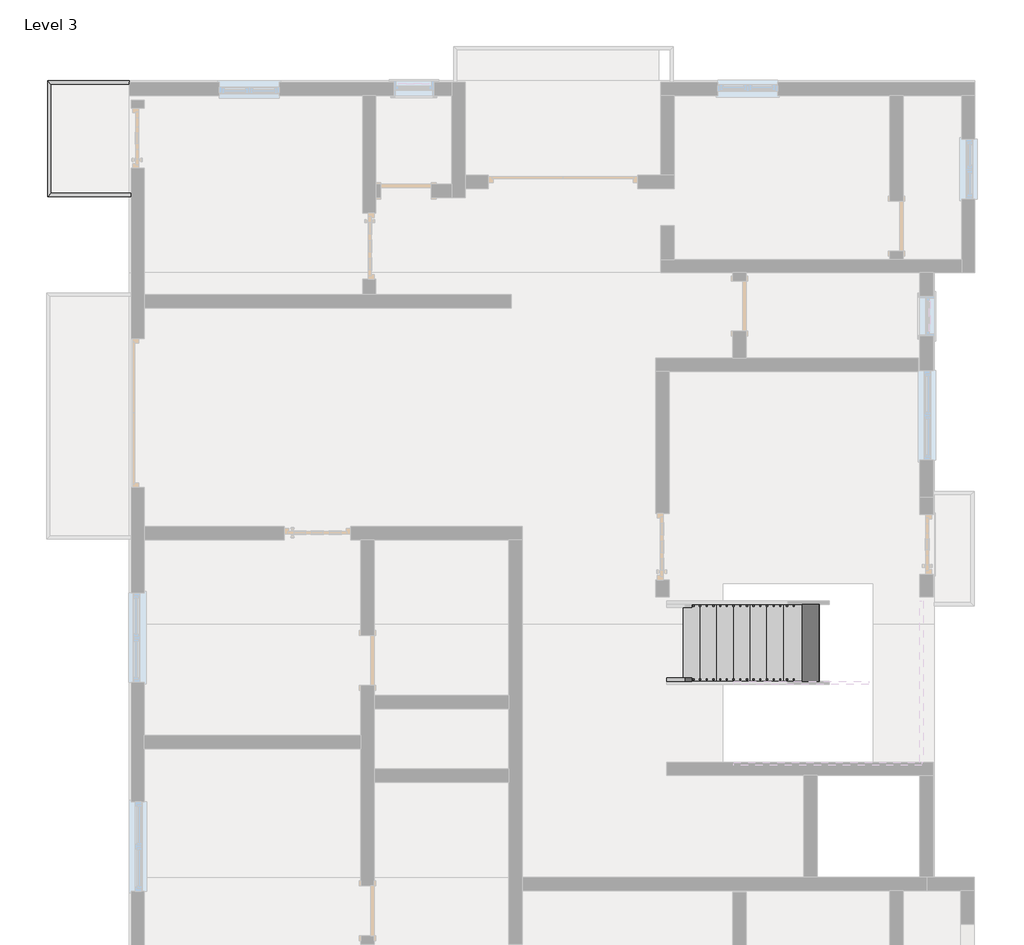
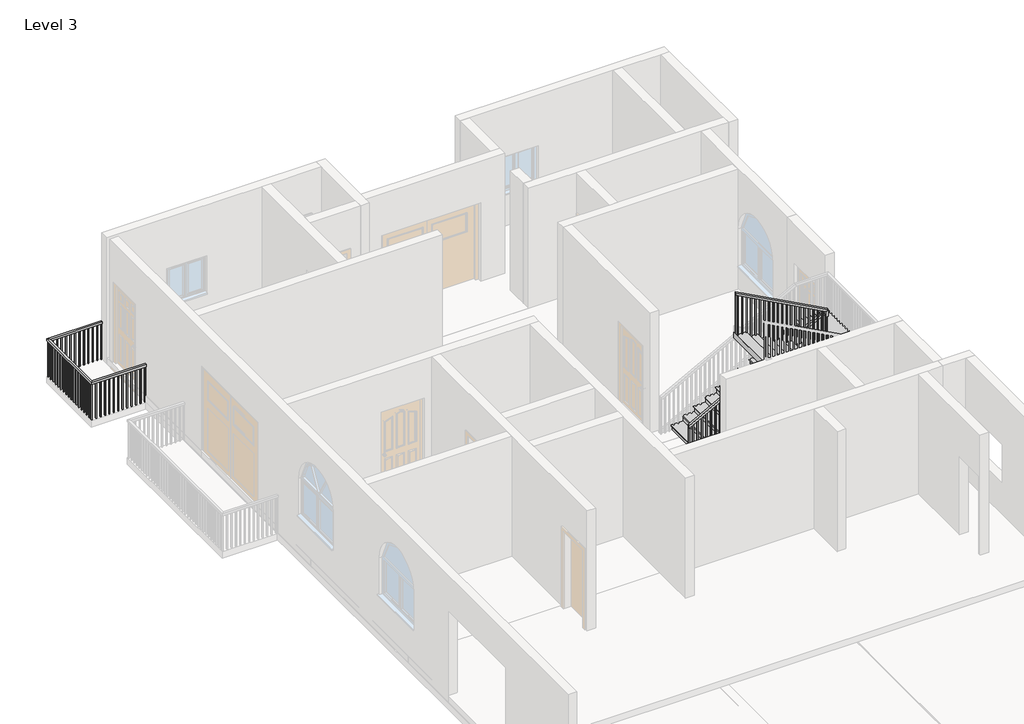
# One storey, part 5 of 7: 2 railings, 1 stair flight.
"""IFC4 building model written with IfcOpenShell, lengths in millimetres."""

from ifc_helpers import new_model, si_unit, frame, origin, place, context, project, spatial, polyline, outline, extrude, faceted_brep, transform, mapped, element, save
from components import stair_flight_4668eb62

model = new_model("IFC4")

# Units and contexts
model_context = context("Model", 3, world=origin())
ifc_project = project(units=[si_unit("LENGTHUNIT", "METRE", prefix="MILLI")], contexts=[model_context])

# Site, building, storey
site = spatial("IfcSite", under=ifc_project)
building = spatial("IfcBuilding", under=site)
storey = spatial("IfcBuildingStorey", under=building, Name="Level 3", Elevation=6096.0)

# Railings
placement = place(None, origin())
element("IfcRailing", 1, ObjectType="Handrail - Rectangular", at=placement, inside=storey, context=model_context, shape_type="SolidModel", body=[
    faceted_brep([(-6354.2109037, 9376.4527313, 7010.4), (-6354.2109037, 9376.4527313, 6959.6), (-6354.2109037, 9427.2527313, 6959.6), (-6354.2109037, 9427.2527313, 7010.4), (-7548.0109037, 9376.4527313, 7010.4), (-7548.0109037, 9376.4527313, 6959.6), (-7598.8109037, 9427.2527313, 6959.6), (-7598.8109037, 9427.2527313, 7010.4), (-7548.0109037, 7717.9584215, 7010.4), (-7548.0109037, 7717.9584215, 6959.6), (-7598.8109037, 7667.1584215, 6959.6), (-7598.8109037, 7667.1584215, 7010.4), (-6330.8013636, 7717.9584215, 7010.4), (-6330.8013636, 7667.1584215, 7010.4), (-6330.8013636, 7667.1584215, 6959.6), (-6330.8013636, 7717.9584215, 6959.6)], [[[0, 1, 2, 3]], [[1, 0, 4, 5]], [[2, 1, 5, 6]], [[3, 2, 6, 7]], [[0, 3, 7, 4]], [[5, 4, 8, 9]], [[6, 5, 9, 10]], [[7, 6, 10, 11]], [[4, 7, 11, 8]], [[12, 13, 14, 15]], [[9, 8, 12, 15]], [[10, 9, 15, 14]], [[11, 10, 14, 13]], [[8, 11, 13, 12]]]),
    extrude(outline(polyline([(-6363.7359037, 7683.0334215), (-6363.7359037, 7702.0834215), (-6344.6859037, 7702.0834215), (-6344.6859037, 7683.0334215), (-6363.7359037, 7683.0334215)])), frame((0.0, 0.0, 6096.0), z_axis=(0.0, 0.0, 1.0), x_axis=(1.0, 0.0, 0.0)), (0.0, 0.0, 1.0), 863.6),
    extrude(outline(polyline([(-6465.3359037, 7683.0334215), (-6465.3359037, 7702.0834215), (-6446.2859037, 7702.0834215), (-6446.2859037, 7683.0334215), (-6465.3359037, 7683.0334215)])), frame((0.0, 0.0, 6096.0), z_axis=(0.0, 0.0, 1.0), x_axis=(1.0, 0.0, 0.0)), (0.0, 0.0, 1.0), 863.6),
    extrude(outline(polyline([(-6566.9359037, 7683.0334215), (-6566.9359037, 7702.0834215), (-6547.8859037, 7702.0834215), (-6547.8859037, 7683.0334215), (-6566.9359037, 7683.0334215)])), frame((0.0, 0.0, 6096.0), z_axis=(0.0, 0.0, 1.0), x_axis=(1.0, 0.0, 0.0)), (0.0, 0.0, 1.0), 863.6),
    extrude(outline(polyline([(-6668.5359037, 7683.0334215), (-6668.5359037, 7702.0834215), (-6649.4859037, 7702.0834215), (-6649.4859037, 7683.0334215), (-6668.5359037, 7683.0334215)])), frame((0.0, 0.0, 6096.0), z_axis=(0.0, 0.0, 1.0), x_axis=(1.0, 0.0, 0.0)), (0.0, 0.0, 1.0), 863.6),
    extrude(outline(polyline([(-6770.1359037, 7683.0334215), (-6770.1359037, 7702.0834215), (-6751.0859037, 7702.0834215), (-6751.0859037, 7683.0334215), (-6770.1359037, 7683.0334215)])), frame((0.0, 0.0, 6096.0), z_axis=(0.0, 0.0, 1.0), x_axis=(1.0, 0.0, 0.0)), (0.0, 0.0, 1.0), 863.6),
    extrude(outline(polyline([(-6871.7359037, 7683.0334215), (-6871.7359037, 7702.0834215), (-6852.6859037, 7702.0834215), (-6852.6859037, 7683.0334215), (-6871.7359037, 7683.0334215)])), frame((0.0, 0.0, 6096.0), z_axis=(0.0, 0.0, 1.0), x_axis=(1.0, 0.0, 0.0)), (0.0, 0.0, 1.0), 863.6),
    extrude(outline(polyline([(-6973.3359037, 7683.0334215), (-6973.3359037, 7702.0834215), (-6954.2859037, 7702.0834215), (-6954.2859037, 7683.0334215), (-6973.3359037, 7683.0334215)])), frame((0.0, 0.0, 6096.0), z_axis=(0.0, 0.0, 1.0), x_axis=(1.0, 0.0, 0.0)), (0.0, 0.0, 1.0), 863.6),
    extrude(outline(polyline([(-7074.9359037, 7683.0334215), (-7074.9359037, 7702.0834215), (-7055.8859037, 7702.0834215), (-7055.8859037, 7683.0334215), (-7074.9359037, 7683.0334215)])), frame((0.0, 0.0, 6096.0), z_axis=(0.0, 0.0, 1.0), x_axis=(1.0, 0.0, 0.0)), (0.0, 0.0, 1.0), 863.6),
    extrude(outline(polyline([(-7176.5359037, 7683.0334215), (-7176.5359037, 7702.0834215), (-7157.4859037, 7702.0834215), (-7157.4859037, 7683.0334215), (-7176.5359037, 7683.0334215)])), frame((0.0, 0.0, 6096.0), z_axis=(0.0, 0.0, 1.0), x_axis=(1.0, 0.0, 0.0)), (0.0, 0.0, 1.0), 863.6),
    extrude(outline(polyline([(-7278.1359037, 7683.0334215), (-7278.1359037, 7702.0834215), (-7259.0859037, 7702.0834215), (-7259.0859037, 7683.0334215), (-7278.1359037, 7683.0334215)])), frame((0.0, 0.0, 6096.0), z_axis=(0.0, 0.0, 1.0), x_axis=(1.0, 0.0, 0.0)), (0.0, 0.0, 1.0), 863.6),
    extrude(outline(polyline([(-7379.7359037, 7683.0334215), (-7379.7359037, 7702.0834215), (-7360.6859037, 7702.0834215), (-7360.6859037, 7683.0334215), (-7379.7359037, 7683.0334215)])), frame((0.0, 0.0, 6096.0), z_axis=(0.0, 0.0, 1.0), x_axis=(1.0, 0.0, 0.0)), (0.0, 0.0, 1.0), 863.6),
    extrude(outline(polyline([(-7481.3359037, 7683.0334215), (-7481.3359037, 7702.0834215), (-7462.2859037, 7702.0834215), (-7462.2859037, 7683.0334215), (-7481.3359037, 7683.0334215)])), frame((0.0, 0.0, 6096.0), z_axis=(0.0, 0.0, 1.0), x_axis=(1.0, 0.0, 0.0)), (0.0, 0.0, 1.0), 863.6),
    extrude(outline(polyline([(-7582.9359037, 7785.7777313), (-7563.8859037, 7785.7777313), (-7563.8859037, 7766.7277313), (-7582.9359037, 7766.7277313), (-7582.9359037, 7785.7777313)])), frame((0.0, 0.0, 6096.0), z_axis=(0.0, 0.0, 1.0), x_axis=(1.0, 0.0, 0.0)), (0.0, 0.0, 1.0), 863.6),
    extrude(outline(polyline([(-7582.9359037, 7887.3777313), (-7563.8859037, 7887.3777313), (-7563.8859037, 7868.3277313), (-7582.9359037, 7868.3277313), (-7582.9359037, 7887.3777313)])), frame((0.0, 0.0, 6096.0), z_axis=(0.0, 0.0, 1.0), x_axis=(1.0, 0.0, 0.0)), (0.0, 0.0, 1.0), 863.6),
    extrude(outline(polyline([(-7582.9359037, 7988.9777313), (-7563.8859037, 7988.9777313), (-7563.8859037, 7969.9277313), (-7582.9359037, 7969.9277313), (-7582.9359037, 7988.9777313)])), frame((0.0, 0.0, 6096.0), z_axis=(0.0, 0.0, 1.0), x_axis=(1.0, 0.0, 0.0)), (0.0, 0.0, 1.0), 863.6),
    extrude(outline(polyline([(-7582.9359037, 8090.5777313), (-7563.8859037, 8090.5777313), (-7563.8859037, 8071.5277313), (-7582.9359037, 8071.5277313), (-7582.9359037, 8090.5777313)])), frame((0.0, 0.0, 6096.0), z_axis=(0.0, 0.0, 1.0), x_axis=(1.0, 0.0, 0.0)), (0.0, 0.0, 1.0), 863.6),
    extrude(outline(polyline([(-7582.9359037, 8192.1777313), (-7563.8859037, 8192.1777313), (-7563.8859037, 8173.1277313), (-7582.9359037, 8173.1277313), (-7582.9359037, 8192.1777313)])), frame((0.0, 0.0, 6096.0), z_axis=(0.0, 0.0, 1.0), x_axis=(1.0, 0.0, 0.0)), (0.0, 0.0, 1.0), 863.6),
    extrude(outline(polyline([(-7582.9359037, 8293.7777313), (-7563.8859037, 8293.7777313), (-7563.8859037, 8274.7277313), (-7582.9359037, 8274.7277313), (-7582.9359037, 8293.7777313)])), frame((0.0, 0.0, 6096.0), z_axis=(0.0, 0.0, 1.0), x_axis=(1.0, 0.0, 0.0)), (0.0, 0.0, 1.0), 863.6),
    extrude(outline(polyline([(-7582.9359037, 8395.3777313), (-7563.8859037, 8395.3777313), (-7563.8859037, 8376.3277313), (-7582.9359037, 8376.3277313), (-7582.9359037, 8395.3777313)])), frame((0.0, 0.0, 6096.0), z_axis=(0.0, 0.0, 1.0), x_axis=(1.0, 0.0, 0.0)), (0.0, 0.0, 1.0), 863.6),
    extrude(outline(polyline([(-7582.9359037, 8496.9777313), (-7563.8859037, 8496.9777313), (-7563.8859037, 8477.9277313), (-7582.9359037, 8477.9277313), (-7582.9359037, 8496.9777313)])), frame((0.0, 0.0, 6096.0), z_axis=(0.0, 0.0, 1.0), x_axis=(1.0, 0.0, 0.0)), (0.0, 0.0, 1.0), 863.6),
    extrude(outline(polyline([(-7582.9359037, 8598.5777313), (-7563.8859037, 8598.5777313), (-7563.8859037, 8579.5277313), (-7582.9359037, 8579.5277313), (-7582.9359037, 8598.5777313)])), frame((0.0, 0.0, 6096.0), z_axis=(0.0, 0.0, 1.0), x_axis=(1.0, 0.0, 0.0)), (0.0, 0.0, 1.0), 863.6),
    extrude(outline(polyline([(-7582.9359037, 8700.1777313), (-7563.8859037, 8700.1777313), (-7563.8859037, 8681.1277313), (-7582.9359037, 8681.1277313), (-7582.9359037, 8700.1777313)])), frame((0.0, 0.0, 6096.0), z_axis=(0.0, 0.0, 1.0), x_axis=(1.0, 0.0, 0.0)), (0.0, 0.0, 1.0), 863.6),
    extrude(outline(polyline([(-7582.9359037, 8801.7777313), (-7563.8859037, 8801.7777313), (-7563.8859037, 8782.7277313), (-7582.9359037, 8782.7277313), (-7582.9359037, 8801.7777313)])), frame((0.0, 0.0, 6096.0), z_axis=(0.0, 0.0, 1.0), x_axis=(1.0, 0.0, 0.0)), (0.0, 0.0, 1.0), 863.6),
    extrude(outline(polyline([(-7582.9359037, 8903.3777313), (-7563.8859037, 8903.3777313), (-7563.8859037, 8884.3277313), (-7582.9359037, 8884.3277313), (-7582.9359037, 8903.3777313)])), frame((0.0, 0.0, 6096.0), z_axis=(0.0, 0.0, 1.0), x_axis=(1.0, 0.0, 0.0)), (0.0, 0.0, 1.0), 863.6),
    extrude(outline(polyline([(-7582.9359037, 9004.9777313), (-7563.8859037, 9004.9777313), (-7563.8859037, 8985.9277313), (-7582.9359037, 8985.9277313), (-7582.9359037, 9004.9777313)])), frame((0.0, 0.0, 6096.0), z_axis=(0.0, 0.0, 1.0), x_axis=(1.0, 0.0, 0.0)), (0.0, 0.0, 1.0), 863.6),
    extrude(outline(polyline([(-7582.9359037, 9106.5777313), (-7563.8859037, 9106.5777313), (-7563.8859037, 9087.5277313), (-7582.9359037, 9087.5277313), (-7582.9359037, 9106.5777313)])), frame((0.0, 0.0, 6096.0), z_axis=(0.0, 0.0, 1.0), x_axis=(1.0, 0.0, 0.0)), (0.0, 0.0, 1.0), 863.6),
    extrude(outline(polyline([(-7582.9359037, 9208.1777313), (-7563.8859037, 9208.1777313), (-7563.8859037, 9189.1277313), (-7582.9359037, 9189.1277313), (-7582.9359037, 9208.1777313)])), frame((0.0, 0.0, 6096.0), z_axis=(0.0, 0.0, 1.0), x_axis=(1.0, 0.0, 0.0)), (0.0, 0.0, 1.0), 863.6),
    extrude(outline(polyline([(-7582.9359037, 9309.7777313), (-7563.8859037, 9309.7777313), (-7563.8859037, 9290.7277313), (-7582.9359037, 9290.7277313), (-7582.9359037, 9309.7777313)])), frame((0.0, 0.0, 6096.0), z_axis=(0.0, 0.0, 1.0), x_axis=(1.0, 0.0, 0.0)), (0.0, 0.0, 1.0), 863.6),
    extrude(outline(polyline([(-7462.2859037, 9411.3777313), (-7462.2859037, 9392.3277313), (-7481.3359037, 9392.3277313), (-7481.3359037, 9411.3777313), (-7462.2859037, 9411.3777313)])), frame((0.0, 0.0, 6096.0), z_axis=(0.0, 0.0, 1.0), x_axis=(1.0, 0.0, 0.0)), (0.0, 0.0, 1.0), 863.6),
    extrude(outline(polyline([(-7360.6859037, 9411.3777313), (-7360.6859037, 9392.3277313), (-7379.7359037, 9392.3277313), (-7379.7359037, 9411.3777313), (-7360.6859037, 9411.3777313)])), frame((0.0, 0.0, 6096.0), z_axis=(0.0, 0.0, 1.0), x_axis=(1.0, 0.0, 0.0)), (0.0, 0.0, 1.0), 863.6),
    extrude(outline(polyline([(-7259.0859037, 9411.3777313), (-7259.0859037, 9392.3277313), (-7278.1359037, 9392.3277313), (-7278.1359037, 9411.3777313), (-7259.0859037, 9411.3777313)])), frame((0.0, 0.0, 6096.0), z_axis=(0.0, 0.0, 1.0), x_axis=(1.0, 0.0, 0.0)), (0.0, 0.0, 1.0), 863.6),
    extrude(outline(polyline([(-7157.4859037, 9411.3777313), (-7157.4859037, 9392.3277313), (-7176.5359037, 9392.3277313), (-7176.5359037, 9411.3777313), (-7157.4859037, 9411.3777313)])), frame((0.0, 0.0, 6096.0), z_axis=(0.0, 0.0, 1.0), x_axis=(1.0, 0.0, 0.0)), (0.0, 0.0, 1.0), 863.6),
    extrude(outline(polyline([(-7055.8859037, 9411.3777313), (-7055.8859037, 9392.3277313), (-7074.9359037, 9392.3277313), (-7074.9359037, 9411.3777313), (-7055.8859037, 9411.3777313)])), frame((0.0, 0.0, 6096.0), z_axis=(0.0, 0.0, 1.0), x_axis=(1.0, 0.0, 0.0)), (0.0, 0.0, 1.0), 863.6),
    extrude(outline(polyline([(-6954.2859037, 9411.3777313), (-6954.2859037, 9392.3277313), (-6973.3359037, 9392.3277313), (-6973.3359037, 9411.3777313), (-6954.2859037, 9411.3777313)])), frame((0.0, 0.0, 6096.0), z_axis=(0.0, 0.0, 1.0), x_axis=(1.0, 0.0, 0.0)), (0.0, 0.0, 1.0), 863.6),
    extrude(outline(polyline([(-6852.6859037, 9411.3777313), (-6852.6859037, 9392.3277313), (-6871.7359037, 9392.3277313), (-6871.7359037, 9411.3777313), (-6852.6859037, 9411.3777313)])), frame((0.0, 0.0, 6096.0), z_axis=(0.0, 0.0, 1.0), x_axis=(1.0, 0.0, 0.0)), (0.0, 0.0, 1.0), 863.6),
    extrude(outline(polyline([(-6751.0859037, 9411.3777313), (-6751.0859037, 9392.3277313), (-6770.1359037, 9392.3277313), (-6770.1359037, 9411.3777313), (-6751.0859037, 9411.3777313)])), frame((0.0, 0.0, 6096.0), z_axis=(0.0, 0.0, 1.0), x_axis=(1.0, 0.0, 0.0)), (0.0, 0.0, 1.0), 863.6),
    extrude(outline(polyline([(-6649.4859037, 9411.3777313), (-6649.4859037, 9392.3277313), (-6668.5359037, 9392.3277313), (-6668.5359037, 9411.3777313), (-6649.4859037, 9411.3777313)])), frame((0.0, 0.0, 6096.0), z_axis=(0.0, 0.0, 1.0), x_axis=(1.0, 0.0, 0.0)), (0.0, 0.0, 1.0), 863.6),
    extrude(outline(polyline([(-6547.8859037, 9411.3777313), (-6547.8859037, 9392.3277313), (-6566.9359037, 9392.3277313), (-6566.9359037, 9411.3777313), (-6547.8859037, 9411.3777313)])), frame((0.0, 0.0, 6096.0), z_axis=(0.0, 0.0, 1.0), x_axis=(1.0, 0.0, 0.0)), (0.0, 0.0, 1.0), 863.6),
    extrude(outline(polyline([(-6446.2859037, 9411.3777313), (-6446.2859037, 9392.3277313), (-6465.3359037, 9392.3277313), (-6465.3359037, 9411.3777313), (-6446.2859037, 9411.3777313)])), frame((0.0, 0.0, 6096.0), z_axis=(0.0, 0.0, 1.0), x_axis=(1.0, 0.0, 0.0)), (0.0, 0.0, 1.0), 863.6),
    extrude(outline(polyline([(-7582.9359037, 7702.0834215), (-7563.8859037, 7702.0834215), (-7563.8859037, 7683.0334215), (-7582.9359037, 7683.0334215), (-7582.9359037, 7702.0834215)])), frame((0.0, 0.0, 6096.0), z_axis=(0.0, 0.0, 1.0), x_axis=(1.0, 0.0, 0.0)), (0.0, 0.0, 1.0), 863.6),
    extrude(outline(polyline([(-7563.8859037, 9411.3777313), (-7563.8859037, 9392.3277313), (-7582.9359037, 9392.3277313), (-7582.9359037, 9411.3777313), (-7563.8859037, 9411.3777313)])), frame((0.0, 0.0, 6096.0), z_axis=(0.0, 0.0, 1.0), x_axis=(1.0, 0.0, 0.0)), (0.0, 0.0, 1.0), 863.6),
    extrude(outline(polyline([(-6349.8513636, 7683.0334215), (-6349.8513636, 7702.0834215), (-6330.8013636, 7702.0834215), (-6330.8013636, 7683.0334215), (-6349.8513636, 7683.0334215)])), frame((0.0, 0.0, 6096.0), z_axis=(0.0, 0.0, 1.0), x_axis=(1.0, 0.0, 0.0)), (0.0, 0.0, 1.0), 863.6),
    extrude(outline(polyline([(-6354.2109037, 9411.3777313), (-6354.2109037, 9392.3277313), (-6373.2609037, 9392.3277313), (-6373.2609037, 9411.3777313), (-6354.2109037, 9411.3777313)])), frame((0.0, 0.0, 6096.0), z_axis=(0.0, 0.0, 1.0), x_axis=(1.0, 0.0, 0.0)), (0.0, 0.0, 1.0), 863.6),
])
element("IfcRailing", 2, ObjectType="Handrail - Rectangular", at=placement, inside=storey, context=model_context, shape_type="SolidModel", body=[
    faceted_brep([(1811.8890963, 347.1962251, 7148.9454545), (1811.8890963, 347.1962251, 7091.1709673), (1811.8890963, 296.3962251, 7091.1709673), (1811.8890963, 296.3962251, 7148.9454545), (4804.8326586, 347.1962251, 8770.2136078), (4855.6326586, 347.1962251, 8739.9573214), (4855.6326586, 296.3962251, 8739.9573214), (4804.8326586, 296.3962251, 8770.2136078), (4804.8326586, 347.1962251, 8811.4909091), (4855.6326586, 347.1962251, 8760.6909091), (4855.6326586, 296.3962251, 8760.6909091), (4804.8326586, 296.3962251, 8811.4909091), (4931.8326586, 347.1962251, 8811.4909091), (4931.8326586, 347.1962251, 8760.6909091), (4881.0326586, 296.3962251, 8760.6909091), (4881.0326586, 296.3962251, 8811.4909091), (4931.8326586, 245.5962251, 8811.4909091), (4881.0326586, 245.5962251, 8811.4909091), (4881.0326586, 194.7962251, 8760.6909091), (4931.8326586, 194.7962251, 8760.6909091)], [[[0, 1, 2, 3]], [[1, 0, 4, 5]], [[2, 1, 5, 6]], [[3, 2, 6, 7]], [[0, 3, 7, 4]], [[5, 4, 8, 9]], [[6, 5, 9, 10]], [[7, 6, 10, 11]], [[4, 7, 11, 8]], [[9, 8, 12, 13]], [[10, 9, 13, 14]], [[11, 10, 14, 15]], [[8, 11, 15, 12]], [[16, 17, 18, 19]], [[13, 12, 16, 19]], [[14, 13, 19, 18]], [[15, 14, 18, 17]], [[12, 15, 17, 16]]]),
    faceted_brep([(4931.8326586, 245.5962251, 8811.4909091), (4931.8326586, 194.7962251, 8760.6909091), (4881.0326586, 194.7962251, 8760.6909091), (4881.0326586, 245.5962251, 8811.4909091), (4931.8326586, 245.5962251, 8922.6126249), (4881.0326586, 245.5962251, 8892.3068093), (4881.0326586, 194.7962251, 8892.3068093), (4931.8326586, 194.7962251, 8922.6126249)], [[[0, 1, 2, 3]], [[4, 5, 6, 7]], [[1, 0, 4, 7]], [[2, 1, 7, 6]], [[3, 2, 6, 5]], [[0, 3, 5, 4]]]),
    faceted_brep([(4931.8326586, 194.7962251, 8922.6126249), (4881.0326586, 194.7962251, 8892.3068093), (4881.0326586, 245.5962251, 8892.3068093), (4931.8326586, 245.5962251, 8922.6126249), (2827.8890963, 194.7962251, 10058.4), (2827.8890963, 245.5962251, 10058.4), (2827.8890963, 245.5962251, 10000.6704456), (2827.8890963, 194.7962251, 10000.6704456)], [[[0, 1, 2, 3]], [[4, 5, 6, 7]], [[1, 0, 4, 7]], [[2, 1, 7, 6]], [[3, 2, 6, 5]], [[0, 3, 5, 4]]]),
    extrude(outline(polyline([(9970.40254, 2883.9576586), (9980.686442, 2864.9076586), (9005.4545455, 2864.9076586), (9005.4545455, 2883.9576586), (9970.40254, 2883.9576586)])), frame((0.0, 210.6712251, 0.0), z_axis=(0.0, 1.0, 0.0), x_axis=(0.0, 0.0, 1.0)), (0.0, 0.0, 1.0), 19.05),
    extrude(outline(polyline([(9915.5550624, 2985.5576586), (9925.8389645, 2966.5076586), (9005.4545455, 2966.5076586), (9005.4545455, 2985.5576586), (9915.5550624, 2985.5576586)])), frame((0.0, 210.6712251, 0.0), z_axis=(0.0, 1.0, 0.0), x_axis=(0.0, 0.0, 1.0)), (0.0, 0.0, 1.0), 19.05),
    extrude(outline(polyline([(9860.7075849, 3087.1576586), (9870.9914869, 3068.1076586), (9005.4545455, 3068.1076586), (9005.4545455, 3087.1576586), (9860.7075849, 3087.1576586)])), frame((0.0, 210.6712251, 0.0), z_axis=(0.0, 1.0, 0.0), x_axis=(0.0, 0.0, 1.0)), (0.0, 0.0, 1.0), 19.05),
    extrude(outline(polyline([(9805.8601073, 3188.7576586), (9816.1440094, 3169.7076586), (8866.9090909, 3169.7076586), (8866.9090909, 3188.7576586), (9805.8601073, 3188.7576586)])), frame((0.0, 210.6712251, 0.0), z_axis=(0.0, 1.0, 0.0), x_axis=(0.0, 0.0, 1.0)), (0.0, 0.0, 1.0), 19.05),
    extrude(outline(polyline([(9751.0126298, 3290.3576586), (9761.2965318, 3271.3076586), (8866.9090909, 3271.3076586), (8866.9090909, 3290.3576586), (9751.0126298, 3290.3576586)])), frame((0.0, 210.6712251, 0.0), z_axis=(0.0, 1.0, 0.0), x_axis=(0.0, 0.0, 1.0)), (0.0, 0.0, 1.0), 19.05),
    extrude(outline(polyline([(9696.1651522, 3391.9576586), (9706.4490542, 3372.9076586), (8728.3636364, 3372.9076586), (8728.3636364, 3391.9576586), (9696.1651522, 3391.9576586)])), frame((0.0, 210.6712251, 0.0), z_axis=(0.0, 1.0, 0.0), x_axis=(0.0, 0.0, 1.0)), (0.0, 0.0, 1.0), 19.05),
    extrude(outline(polyline([(9641.3176746, 3493.5576586), (9651.6015767, 3474.5076586), (8728.3636364, 3474.5076586), (8728.3636364, 3493.5576586), (9641.3176746, 3493.5576586)])), frame((0.0, 210.6712251, 0.0), z_axis=(0.0, 1.0, 0.0), x_axis=(0.0, 0.0, 1.0)), (0.0, 0.0, 1.0), 19.05),
    extrude(outline(polyline([(9586.4701971, 3595.1576586), (9596.7540991, 3576.1076586), (8728.3636364, 3576.1076586), (8728.3636364, 3595.1576586), (9586.4701971, 3595.1576586)])), frame((0.0, 210.6712251, 0.0), z_axis=(0.0, 1.0, 0.0), x_axis=(0.0, 0.0, 1.0)), (0.0, 0.0, 1.0), 19.05),
    extrude(outline(polyline([(9531.6227195, 3696.7576586), (9541.9066216, 3677.7076586), (8589.8181818, 3677.7076586), (8589.8181818, 3696.7576586), (9531.6227195, 3696.7576586)])), frame((0.0, 210.6712251, 0.0), z_axis=(0.0, 1.0, 0.0), x_axis=(0.0, 0.0, 1.0)), (0.0, 0.0, 1.0), 19.05),
    extrude(outline(polyline([(9476.775242, 3798.3576586), (9487.059144, 3779.3076586), (8589.8181818, 3779.3076586), (8589.8181818, 3798.3576586), (9476.775242, 3798.3576586)])), frame((0.0, 210.6712251, 0.0), z_axis=(0.0, 1.0, 0.0), x_axis=(0.0, 0.0, 1.0)), (0.0, 0.0, 1.0), 19.05),
    extrude(outline(polyline([(9421.9277644, 3899.9576586), (9432.2116665, 3880.9076586), (8451.2727273, 3880.9076586), (8451.2727273, 3899.9576586), (9421.9277644, 3899.9576586)])), frame((0.0, 210.6712251, 0.0), z_axis=(0.0, 1.0, 0.0), x_axis=(0.0, 0.0, 1.0)), (0.0, 0.0, 1.0), 19.05),
    extrude(outline(polyline([(9367.0802869, 4001.5576586), (9377.3641889, 3982.5076586), (8451.2727273, 3982.5076586), (8451.2727273, 4001.5576586), (9367.0802869, 4001.5576586)])), frame((0.0, 210.6712251, 0.0), z_axis=(0.0, 1.0, 0.0), x_axis=(0.0, 0.0, 1.0)), (0.0, 0.0, 1.0), 19.05),
    extrude(outline(polyline([(9312.2328093, 4103.1576586), (9322.5167113, 4084.1076586), (8451.2727273, 4084.1076586), (8451.2727273, 4103.1576586), (9312.2328093, 4103.1576586)])), frame((0.0, 210.6712251, 0.0), z_axis=(0.0, 1.0, 0.0), x_axis=(0.0, 0.0, 1.0)), (0.0, 0.0, 1.0), 19.05),
    extrude(outline(polyline([(9257.3853317, 4204.7576586), (9267.6692338, 4185.7076586), (8312.7272727, 4185.7076586), (8312.7272727, 4204.7576586), (9257.3853317, 4204.7576586)])), frame((0.0, 210.6712251, 0.0), z_axis=(0.0, 1.0, 0.0), x_axis=(0.0, 0.0, 1.0)), (0.0, 0.0, 1.0), 19.05),
    extrude(outline(polyline([(9202.5378542, 4306.3576586), (9212.8217562, 4287.3076586), (8312.7272727, 4287.3076586), (8312.7272727, 4306.3576586), (9202.5378542, 4306.3576586)])), frame((0.0, 210.6712251, 0.0), z_axis=(0.0, 1.0, 0.0), x_axis=(0.0, 0.0, 1.0)), (0.0, 0.0, 1.0), 19.05),
    extrude(outline(polyline([(9147.6903766, 4407.9576586), (9157.9742787, 4388.9076586), (8174.1818182, 4388.9076586), (8174.1818182, 4407.9576586), (9147.6903766, 4407.9576586)])), frame((0.0, 210.6712251, 0.0), z_axis=(0.0, 1.0, 0.0), x_axis=(0.0, 0.0, 1.0)), (0.0, 0.0, 1.0), 19.05),
    extrude(outline(polyline([(9092.8428991, 4509.5576586), (9103.1268011, 4490.5076586), (8174.1818182, 4490.5076586), (8174.1818182, 4509.5576586), (9092.8428991, 4509.5576586)])), frame((0.0, 210.6712251, 0.0), z_axis=(0.0, 1.0, 0.0), x_axis=(0.0, 0.0, 1.0)), (0.0, 0.0, 1.0), 19.05),
    extrude(outline(polyline([(9037.9954215, 4611.1576586), (9048.2793236, 4592.1076586), (8174.1818182, 4592.1076586), (8174.1818182, 4611.1576586), (9037.9954215, 4611.1576586)])), frame((0.0, 210.6712251, 0.0), z_axis=(0.0, 1.0, 0.0), x_axis=(0.0, 0.0, 1.0)), (0.0, 0.0, 1.0), 19.05),
    extrude(outline(polyline([(8983.147944, 4712.7576586), (8993.431846, 4693.7076586), (8035.6363636, 4693.7076586), (8035.6363636, 4712.7576586), (8983.147944, 4712.7576586)])), frame((0.0, 210.6712251, 0.0), z_axis=(0.0, 1.0, 0.0), x_axis=(0.0, 0.0, 1.0)), (0.0, 0.0, 1.0), 19.05),
    extrude(outline(polyline([(8928.3004664, 4814.3576586), (8938.5843684, 4795.3076586), (8035.6363636, 4795.3076586), (8035.6363636, 4814.3576586), (8928.3004664, 4814.3576586)])), frame((0.0, 210.6712251, 0.0), z_axis=(0.0, 1.0, 0.0), x_axis=(0.0, 0.0, 1.0)), (0.0, 0.0, 1.0), 19.05),
    extrude(outline(polyline([(4850.3640963, 312.2712251), (4850.3640963, 331.3212251), (4869.4140963, 331.3212251), (4869.4140963, 312.2712251), (4850.3640963, 312.2712251)])), frame((0.0, 0.0, 7758.5454545), z_axis=(0.0, 0.0, 1.0), x_axis=(1.0, 0.0, 0.0)), (0.0, 0.0, 1.0), 1002.1454545),
    extrude(outline(polyline([(8692.3862812, 4767.8140963), (8682.0669559, 4748.7640963), (7758.5454545, 4748.7640963), (7758.5454545, 4767.8140963), (8692.3862812, 4767.8140963)])), frame((0.0, 312.2712251, 0.0), z_axis=(0.0, 1.0, 0.0), x_axis=(0.0, 0.0, 1.0)), (0.0, 0.0, 1.0), 19.05),
    extrude(outline(polyline([(8637.3498795, 4666.2140963), (8627.0305541, 4647.1640963), (7758.5454545, 4647.1640963), (7758.5454545, 4666.2140963), (8637.3498795, 4666.2140963)])), frame((0.0, 312.2712251, 0.0), z_axis=(0.0, 1.0, 0.0), x_axis=(0.0, 0.0, 1.0)), (0.0, 0.0, 1.0), 19.05),
    extrude(outline(polyline([(8582.3134777, 4564.6140963), (8571.9941524, 4545.5640963), (7620.0, 4545.5640963), (7620.0, 4564.6140963), (8582.3134777, 4564.6140963)])), frame((0.0, 312.2712251, 0.0), z_axis=(0.0, 1.0, 0.0), x_axis=(0.0, 0.0, 1.0)), (0.0, 0.0, 1.0), 19.05),
    extrude(outline(polyline([(8527.2770759, 4463.0140963), (8516.9577506, 4443.9640963), (7620.0, 4443.9640963), (7620.0, 4463.0140963), (8527.2770759, 4463.0140963)])), frame((0.0, 312.2712251, 0.0), z_axis=(0.0, 1.0, 0.0), x_axis=(0.0, 0.0, 1.0)), (0.0, 0.0, 1.0), 19.05),
    extrude(outline(polyline([(8472.2406742, 4361.4140963), (8461.9213488, 4342.3640963), (7620.0, 4342.3640963), (7620.0, 4361.4140963), (8472.2406742, 4361.4140963)])), frame((0.0, 312.2712251, 0.0), z_axis=(0.0, 1.0, 0.0), x_axis=(0.0, 0.0, 1.0)), (0.0, 0.0, 1.0), 19.05),
    extrude(outline(polyline([(8417.2042724, 4259.8140963), (8406.8849471, 4240.7640963), (7481.4545455, 4240.7640963), (7481.4545455, 4259.8140963), (8417.2042724, 4259.8140963)])), frame((0.0, 312.2712251, 0.0), z_axis=(0.0, 1.0, 0.0), x_axis=(0.0, 0.0, 1.0)), (0.0, 0.0, 1.0), 19.05),
    extrude(outline(polyline([(8362.1678706, 4158.2140963), (8351.8485453, 4139.1640963), (7481.4545455, 4139.1640963), (7481.4545455, 4158.2140963), (8362.1678706, 4158.2140963)])), frame((0.0, 312.2712251, 0.0), z_axis=(0.0, 1.0, 0.0), x_axis=(0.0, 0.0, 1.0)), (0.0, 0.0, 1.0), 19.05),
    extrude(outline(polyline([(8307.1314688, 4056.6140963), (8296.8121435, 4037.5640963), (7342.9090909, 4037.5640963), (7342.9090909, 4056.6140963), (8307.1314688, 4056.6140963)])), frame((0.0, 312.2712251, 0.0), z_axis=(0.0, 1.0, 0.0), x_axis=(0.0, 0.0, 1.0)), (0.0, 0.0, 1.0), 19.05),
    extrude(outline(polyline([(8252.0950671, 3955.0140963), (8241.7757417, 3935.9640963), (7342.9090909, 3935.9640963), (7342.9090909, 3955.0140963), (8252.0950671, 3955.0140963)])), frame((0.0, 312.2712251, 0.0), z_axis=(0.0, 1.0, 0.0), x_axis=(0.0, 0.0, 1.0)), (0.0, 0.0, 1.0), 19.05),
    extrude(outline(polyline([(8197.0586653, 3853.4140963), (8186.73934, 3834.3640963), (7342.9090909, 3834.3640963), (7342.9090909, 3853.4140963), (8197.0586653, 3853.4140963)])), frame((0.0, 312.2712251, 0.0), z_axis=(0.0, 1.0, 0.0), x_axis=(0.0, 0.0, 1.0)), (0.0, 0.0, 1.0), 19.05),
    extrude(outline(polyline([(8142.0222635, 3751.8140963), (8131.7029382, 3732.7640963), (7204.3636364, 3732.7640963), (7204.3636364, 3751.8140963), (8142.0222635, 3751.8140963)])), frame((0.0, 312.2712251, 0.0), z_axis=(0.0, 1.0, 0.0), x_axis=(0.0, 0.0, 1.0)), (0.0, 0.0, 1.0), 19.05),
    extrude(outline(polyline([(8086.9858618, 3650.2140963), (8076.6665364, 3631.1640963), (7204.3636364, 3631.1640963), (7204.3636364, 3650.2140963), (8086.9858618, 3650.2140963)])), frame((0.0, 312.2712251, 0.0), z_axis=(0.0, 1.0, 0.0), x_axis=(0.0, 0.0, 1.0)), (0.0, 0.0, 1.0), 19.05),
    extrude(outline(polyline([(8031.94946, 3548.6140963), (8021.6301347, 3529.5640963), (7065.8181818, 3529.5640963), (7065.8181818, 3548.6140963), (8031.94946, 3548.6140963)])), frame((0.0, 312.2712251, 0.0), z_axis=(0.0, 1.0, 0.0), x_axis=(0.0, 0.0, 1.0)), (0.0, 0.0, 1.0), 19.05),
    extrude(outline(polyline([(7976.9130582, 3447.0140963), (7966.5937329, 3427.9640963), (7065.8181818, 3427.9640963), (7065.8181818, 3447.0140963), (7976.9130582, 3447.0140963)])), frame((0.0, 312.2712251, 0.0), z_axis=(0.0, 1.0, 0.0), x_axis=(0.0, 0.0, 1.0)), (0.0, 0.0, 1.0), 19.05),
    extrude(outline(polyline([(7921.8766565, 3345.4140963), (7911.5573311, 3326.3640963), (7065.8181818, 3326.3640963), (7065.8181818, 3345.4140963), (7921.8766565, 3345.4140963)])), frame((0.0, 312.2712251, 0.0), z_axis=(0.0, 1.0, 0.0), x_axis=(0.0, 0.0, 1.0)), (0.0, 0.0, 1.0), 19.05),
    extrude(outline(polyline([(7866.8402547, 3243.8140963), (7856.5209294, 3224.7640963), (6927.2727273, 3224.7640963), (6927.2727273, 3243.8140963), (7866.8402547, 3243.8140963)])), frame((0.0, 312.2712251, 0.0), z_axis=(0.0, 1.0, 0.0), x_axis=(0.0, 0.0, 1.0)), (0.0, 0.0, 1.0), 19.05),
    extrude(outline(polyline([(7811.8038529, 3142.2140963), (7801.4845276, 3123.1640963), (6927.2727273, 3123.1640963), (6927.2727273, 3142.2140963), (7811.8038529, 3142.2140963)])), frame((0.0, 312.2712251, 0.0), z_axis=(0.0, 1.0, 0.0), x_axis=(0.0, 0.0, 1.0)), (0.0, 0.0, 1.0), 19.05),
    extrude(outline(polyline([(7756.7674512, 3040.6140963), (7746.4481258, 3021.5640963), (6788.7272727, 3021.5640963), (6788.7272727, 3040.6140963), (7756.7674512, 3040.6140963)])), frame((0.0, 312.2712251, 0.0), z_axis=(0.0, 1.0, 0.0), x_axis=(0.0, 0.0, 1.0)), (0.0, 0.0, 1.0), 19.05),
    extrude(outline(polyline([(7701.7310494, 2939.0140963), (7691.4117241, 2919.9640963), (6788.7272727, 2919.9640963), (6788.7272727, 2939.0140963), (7701.7310494, 2939.0140963)])), frame((0.0, 312.2712251, 0.0), z_axis=(0.0, 1.0, 0.0), x_axis=(0.0, 0.0, 1.0)), (0.0, 0.0, 1.0), 19.05),
    extrude(outline(polyline([(7646.6946476, 2837.4140963), (7636.3753223, 2818.3640963), (6788.7272727, 2818.3640963), (6788.7272727, 2837.4140963), (7646.6946476, 2837.4140963)])), frame((0.0, 312.2712251, 0.0), z_axis=(0.0, 1.0, 0.0), x_axis=(0.0, 0.0, 1.0)), (0.0, 0.0, 1.0), 19.05),
    extrude(outline(polyline([(7591.6582459, 2735.8140963), (7581.3389205, 2716.7640963), (6650.1818182, 2716.7640963), (6650.1818182, 2735.8140963), (7591.6582459, 2735.8140963)])), frame((0.0, 312.2712251, 0.0), z_axis=(0.0, 1.0, 0.0), x_axis=(0.0, 0.0, 1.0)), (0.0, 0.0, 1.0), 19.05),
    extrude(outline(polyline([(7536.6218441, 2634.2140963), (7526.3025188, 2615.1640963), (6650.1818182, 2615.1640963), (6650.1818182, 2634.2140963), (7536.6218441, 2634.2140963)])), frame((0.0, 312.2712251, 0.0), z_axis=(0.0, 1.0, 0.0), x_axis=(0.0, 0.0, 1.0)), (0.0, 0.0, 1.0), 19.05),
    extrude(outline(polyline([(7481.5854423, 2532.6140963), (7471.266117, 2513.5640963), (6511.6363636, 2513.5640963), (6511.6363636, 2532.6140963), (7481.5854423, 2532.6140963)])), frame((0.0, 312.2712251, 0.0), z_axis=(0.0, 1.0, 0.0), x_axis=(0.0, 0.0, 1.0)), (0.0, 0.0, 1.0), 19.05),
    extrude(outline(polyline([(7426.5490405, 2431.0140963), (7416.2297152, 2411.9640963), (6511.6363636, 2411.9640963), (6511.6363636, 2431.0140963), (7426.5490405, 2431.0140963)])), frame((0.0, 312.2712251, 0.0), z_axis=(0.0, 1.0, 0.0), x_axis=(0.0, 0.0, 1.0)), (0.0, 0.0, 1.0), 19.05),
    extrude(outline(polyline([(7371.5126388, 2329.4140963), (7361.1933134, 2310.3640963), (6511.6363636, 2310.3640963), (6511.6363636, 2329.4140963), (7371.5126388, 2329.4140963)])), frame((0.0, 312.2712251, 0.0), z_axis=(0.0, 1.0, 0.0), x_axis=(0.0, 0.0, 1.0)), (0.0, 0.0, 1.0), 19.05),
    extrude(outline(polyline([(7316.476237, 2227.8140963), (7306.1569117, 2208.7640963), (6373.0909091, 2208.7640963), (6373.0909091, 2227.8140963), (7316.476237, 2227.8140963)])), frame((0.0, 312.2712251, 0.0), z_axis=(0.0, 1.0, 0.0), x_axis=(0.0, 0.0, 1.0)), (0.0, 0.0, 1.0), 19.05),
    extrude(outline(polyline([(7261.4398352, 2126.2140963), (7251.1205099, 2107.1640963), (6373.0909091, 2107.1640963), (6373.0909091, 2126.2140963), (7261.4398352, 2126.2140963)])), frame((0.0, 312.2712251, 0.0), z_axis=(0.0, 1.0, 0.0), x_axis=(0.0, 0.0, 1.0)), (0.0, 0.0, 1.0), 19.05),
    extrude(outline(polyline([(7206.4034335, 2024.6140963), (7196.0841081, 2005.5640963), (6234.5454545, 2005.5640963), (6234.5454545, 2024.6140963), (7206.4034335, 2024.6140963)])), frame((0.0, 312.2712251, 0.0), z_axis=(0.0, 1.0, 0.0), x_axis=(0.0, 0.0, 1.0)), (0.0, 0.0, 1.0), 19.05),
    extrude(outline(polyline([(7151.3670317, 1923.0140963), (7141.0477064, 1903.9640963), (6234.5454545, 1903.9640963), (6234.5454545, 1923.0140963), (7151.3670317, 1923.0140963)])), frame((0.0, 312.2712251, 0.0), z_axis=(0.0, 1.0, 0.0), x_axis=(0.0, 0.0, 1.0)), (0.0, 0.0, 1.0), 19.05),
    extrude(outline(polyline([(4896.9076586, 229.7212251), (4915.9576586, 229.7212251), (4915.9576586, 210.6712251), (4896.9076586, 210.6712251), (4896.9076586, 229.7212251)])), frame((0.0, 0.0, 7897.0909091), z_axis=(0.0, 0.0, 1.0), x_axis=(1.0, 0.0, 0.0)), (0.0, 0.0, 1.0), 863.6),
    extrude(outline(polyline([(4896.9076586, 312.2712251), (4896.9076586, 331.3212251), (4915.9576586, 331.3212251), (4915.9576586, 312.2712251), (4896.9076586, 312.2712251)])), frame((0.0, 0.0, 7897.0909091), z_axis=(0.0, 0.0, 1.0), x_axis=(1.0, 0.0, 0.0)), (0.0, 0.0, 1.0), 863.6),
    extrude(outline(polyline([(9990.3865436, 2846.9390963), (10000.6704456, 2827.8890963), (9005.4545455, 2827.8890963), (9005.4545455, 2846.9390963), (9990.3865436, 2846.9390963)])), frame((0.0, 210.6712251, 0.0), z_axis=(0.0, 1.0, 0.0), x_axis=(0.0, 0.0, 1.0)), (0.0, 0.0, 1.0), 19.05),
    extrude(outline(polyline([(7101.4902926, 1830.9390963), (7091.1709673, 1811.8890963), (6234.5454545, 1811.8890963), (6234.5454545, 1830.9390963), (7101.4902926, 1830.9390963)])), frame((0.0, 312.2712251, 0.0), z_axis=(0.0, 1.0, 0.0), x_axis=(0.0, 0.0, 1.0)), (0.0, 0.0, 1.0), 19.05),
])

# Stair flight
stair_flight_shape = stair_flight_4668eb62(model_context)
element("IfcStairFlight", 3, ObjectType="2\" Tread 1\" Nosing 1/4\" Riser", at=placement, inside=storey, context=model_context, shape_type="MappedRepresentation", body=[
    mapped(stair_flight_shape, transform((0.0, 0.0, 0.0), x_axis=(1.0, 0.0, 0.0), y_axis=(0.0, 1.0, 0.0), z_axis=(0.0, 0.0, 1.0))),
])

save(model, "model.ifc")

# Revit data of these elements
# Type "Handrail - Rectangular"
#   Assembly Code = "C2010400"
#   built-in parameter 1008612 = 0.0416667 (stored number, unit not read)
#   built-in parameter 1008611 = 0.0416667 (stored number, unit not read)
#   built-in parameter 1008609 = 0.333333 (stored number, unit not read)
#   built-in parameter 1008604 = 0.166667 (stored number, unit not read)
#   built-in parameter 1008603 = 0.166667 (stored number, unit not read)
#   Railing Height = 3' - 0"
#   built-in parameter 1008630 = 2
#   built-in parameter 1008610 = 2
#   built-in parameter 1008618 = Baluster - Square : 3/4"
# Elements 1, 2 (IfcRailing, "Handrail - Rectangular")
#   Phase Created = New Construction
# Element 3 (IfcStairFlight, "2\" Tread 1\" Nosing 1/4\" Riser")
#   Phase Created = New Construction
